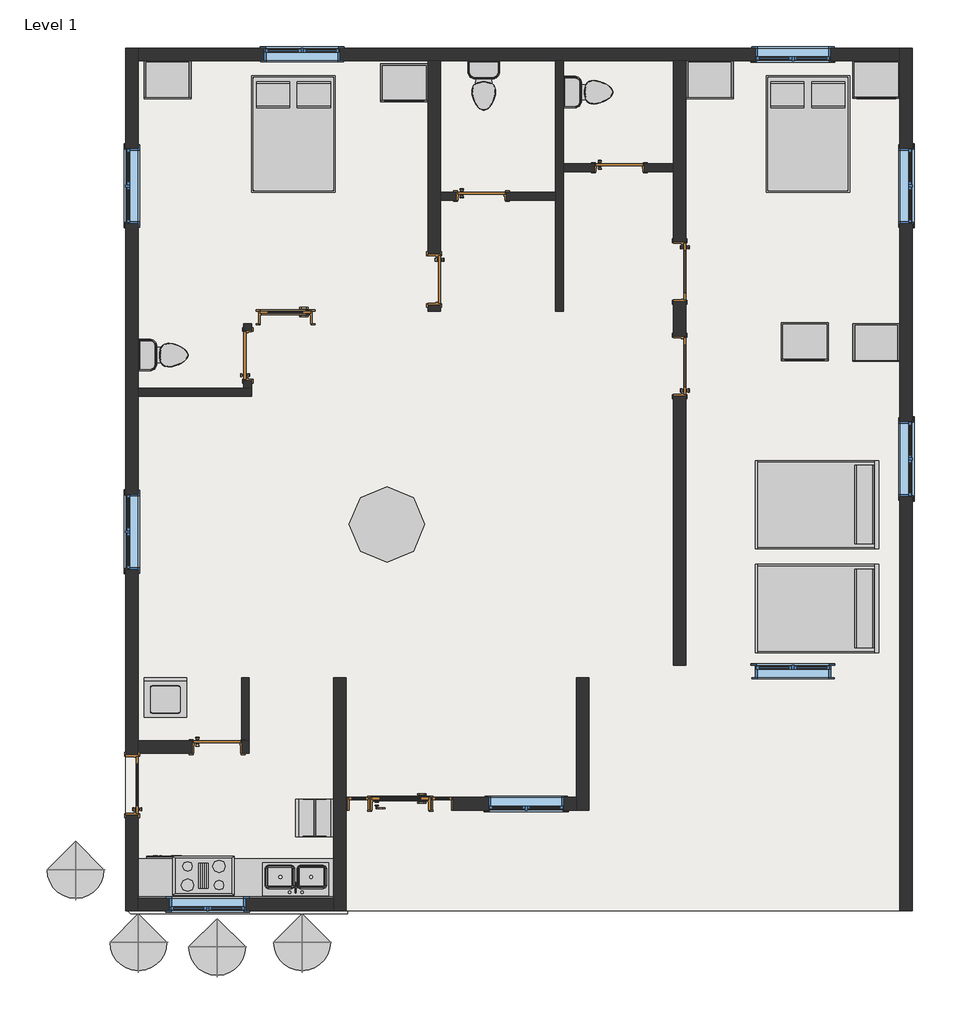
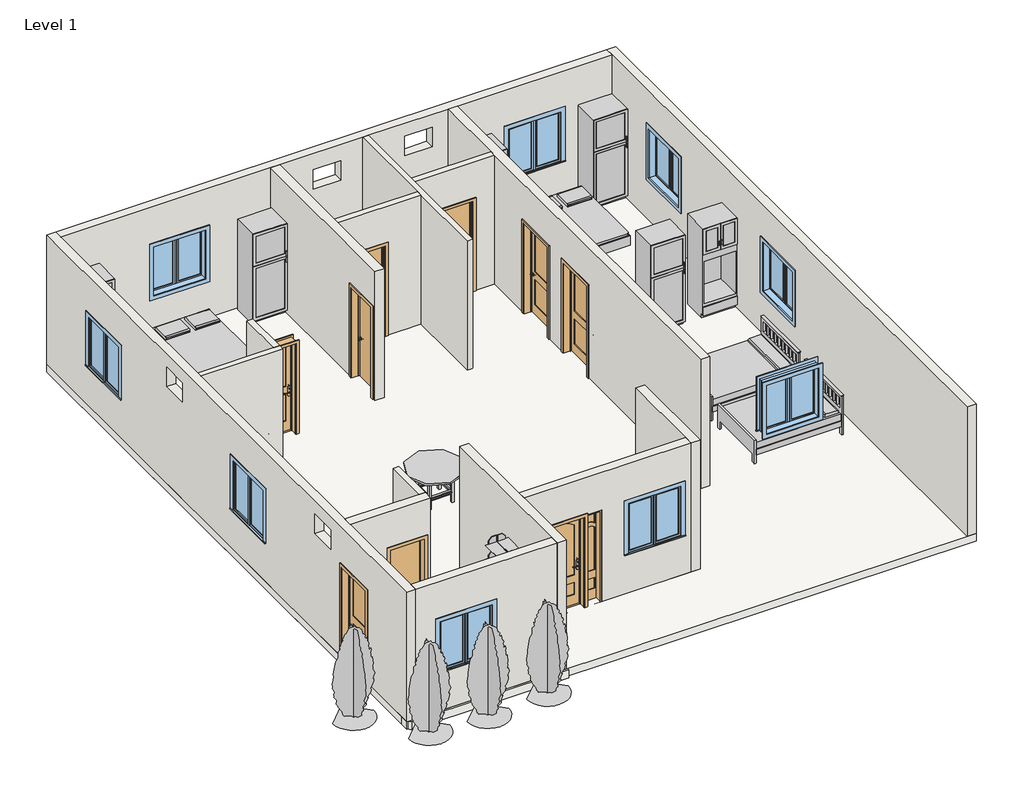
# One storey, incomplete: 16 walls, 13 doors, 12 furniture elements, 9 windows, 4 flow terminals, 4 geographic elements, 4 proxies, 3 slabs.
# Revit data of these elements (continued)
# Element 7 (IfcDoor, "32\" x 84\"") (continued)
#   Materials on its faces: "Cherry", "Aluminum", "Glass"
# Element 8 (IfcDoor, "36\" x 84\"")
#   Threshold Offset = 0' - 0 1/2"
#   Swing Angle = 90.00°
#   Door Offset = 0' - 0"
#   Threshold = yes
#   Exterior Trim = yes
#   Phase Created = New Construction
#   Materials on its faces: "Cherry", "Aluminum", "Glass"
# Elements 9, 10, 11 (IfcDoor, "Door-Interior-Single-2_Panel-Wood : 36\" x 84\"")
#   Swing Angle = 90.00°
#   Phase Created = New Construction
#   Materials on its faces: "Cherry", "Aluminum"
# Elements 12, 13, 14, 15 (IfcDoor, "Door-Interior-Single-Flush_Panel-Wood")
#   Swing Angle = 90.00°
#   Phase Created = New Construction
#   Materials on its faces: "Cherry", "Aluminum"
# Element 16 (IfcDoor, "Door-Interior-Single-Flush_Panel-Wood : 30\" x 84\"")
#   Swing Angle = 90.00°
#   Phase Created = New Construction
#   Materials on its faces: "Cherry", "Aluminum"
# Element 17 (IfcDoor, "Entry Door Handle : Standard")
#   Phase Created = New Construction
#   Materials on its faces: "Aluminum"
# Element 18 (IfcFlowTerminal, "Sink Kitchen-Double : 42\" x 21\"")
#   Mark = "1"
#   Phase Created = New Construction
#   Materials on its faces: "Steel, Polished"
# Element 19 (IfcFlowTerminal, "Toilet-Domestic-3D : Toilet-Domestic-3D")
#   Mark = "2"
#   Phase Created = New Construction
#   Materials on its faces: "Porcelain, Linen", "Laminate, Linen, Matte"
# Element 20 (IfcFlowTerminal, "Toilet-Domestic-3D : Toilet-Domestic-3D")
#   Mark = "3"
#   Phase Created = New Construction
#   Materials on its faces: "Porcelain, Linen", "Laminate, Linen, Matte"
# Element 21 (IfcFlowTerminal, "Toilet-Domestic-3D : Toilet-Domestic-3D")
#   Mark = "4"
#   Phase Created = New Construction
#   Materials on its faces: "Porcelain, Linen", "Laminate, Linen, Matte"
# Elements 22, 23 (IfcFurniture, "Bed-Box : Double 53\" x 74\"")
#   Phase Created = New Construction
#   Materials on its faces: "Birch", "Linen, White"
# Elements 24, 25 (IfcFurniture, "Bed-Shaker : Double 56\" x 78\"")
#   Phase Created = New Construction
#   Materials on its faces: "Birch", "Linen, White"
# Element 26 (IfcFurniture, "Counter Top w Sink : 24\" Depth")
#   Sink Opening Width = 3' - 3"
#   Sink Opening Depth = 1' - 3"
#   Sink Location To Wall = 0' - 6"
#   Sink Location = 2' - 0"
#   Length = 10' - 4"
#   Phase Created = New Construction
#   Materials on its faces: "Counter Top"
# Element 27 (IfcFurniture, "Table-Dining Round w Chairs : 36\" Diameter")
#   Phase Created = New Construction
#   Materials on its faces: "Pine", "Laminate, Linen, Matte"
# Elements 28, 29, 30 (IfcFurniture, "Tall Cabinet-2 Door-Built in : 30\"")
#   Phase Created = New Construction
#   Materials on its faces: "Cabinets", "Cabinets - Handles", "Glass"
# Elements 31, 32, 33 (IfcFurniture, "Tall Cabinet-Single Door(2) : 30\"")
#   Phase Created = New Construction
#   Materials on its faces: "Cabinets", "Cabinets - Handles"
# Elements 34, 35, 36, 37 (IfcGeographicElement, "RPC Tree - Conifer : Chinese Juniper - 7'")
#   Phase Created = New Construction
# Elements 38, 39, 40 (IfcSlab, "Generic - 12\"")
#   Height Offset From Level = 0' - 0"
#   Phase Created = New Construction
#   Materials on its faces: "Plywood, Sheathing"
# Elements 41, 42 (IfcWall)
#   Top Offset = 0' - 0"
#   Base Offset = 0' - 0"
#   Unconnected Height = 10' - 0"
#   wall height = 10' - 0"
#   Phase Created = New Construction
#   Base Constraint = Level 1
#   Materials on its faces: "Birch"
# Elements 43, 44, 45, 46 (IfcWall, "Generic - 5\"")
#   Top Offset = 0' - 0"
#   Base Offset = 0' - 0"
#   Unconnected Height = 10' - 0"
#   wall height = 10' - 0"
#   Phase Created = New Construction
#   Base Constraint = Level 1
#   Materials on its faces: "Default Wall"
# Elements 47, 48 (IfcWall, "Generic - 5\"")
#   Top Offset = 0' - 0"
#   Base Offset = 0' - 0"
#   wall height = 10' - 0"
#   Phase Created = New Construction
#   Base Constraint = Level 1
#   Top Constraint = Level 2
#   Materials on its faces: "Default Wall"
# Elements 49, 50, 52 (IfcWall, "Generic - 8\"")
#   Top Offset = 0' - 0"
#   Base Offset = 0' - 0"
#   Unconnected Height = 10' - 0"
#   wall height = 10' - 0"
#   Phase Created = New Construction
#   Base Constraint = Level 1
#   Materials on its faces: "Default Wall"
# Element 51 (IfcWall, "Generic - 8\"")
#   Top Offset = 0' - 0"
#   Base Offset = 0' - 0"
#   Unconnected Height = 10' - 0"
#   wall height = 10' - 0"
#   Phase Created = New Construction
#   Base Constraint = Level 1
#   Materials on its faces: "Default Wall", "Birch"
# Element 53 (IfcWall, "a")
#   Top Offset = 0' - 0"
#   Base Offset = 0' - 0"
#   Unconnected Height = 10' - 0"
#   wall height = 10' - 0"
#   Phase Created = New Construction
#   Base Constraint = Level 1
#   Materials on its faces: "Birch"
# Element 54 (IfcWall, "aw")
#   Top Offset = 0' - 0"
#   Base Offset = 0' - 0"
#   Unconnected Height = 10' - 0"
#   wall height = 10' - 0"
#   Phase Created = New Construction
#   Base Constraint = Level 1
#   Materials on its faces: "Birch"
# Elements 55, 56 (IfcWall, "dq")
#   Top Offset = 0' - 0"
#   Base Offset = 0' - 0"
#   Unconnected Height = 10' - 0"
#   wall height = 10' - 0"
#   Phase Created = New Construction
#   Base Constraint = Level 1
#   Materials on its faces: "Birch"
# Element 57 (IfcWindow, "Casement Dbl with Trim : 48\" x 48\"")
#   Mark = "3"
#   Phase Created = New Construction
#   Materials on its faces: "Sash", "Trim", "Glass"
# Element 58 (IfcWindow, "Casement Dbl with Trim : 48\" x 48\"")
#   Mark = "4"
#   Phase Created = New Construction
#   Materials on its faces: "Sash", "Trim", "Glass"
# Element 59 (IfcWindow, "Casement Dbl with Trim : 48\" x 48\"")
#   Mark = "2"
#   Phase Created = New Construction
#   Materials on its faces: "Sash", "Trim", "Glass"
# Element 60 (IfcWindow, "Casement Dbl with Trim : 48\" x 48\"")
#   Mark = "1"
#   Phase Created = New Construction
#   Materials on its faces: "Sash", "Trim", "Glass"
# Element 61 (IfcWindow, "Casement Dbl with Trim : 48\" x 48\"")
#   Mark = "7"
#   Phase Created = New Construction
#   Materials on its faces: "Sash", "Trim", "Glass"
# Element 62 (IfcWindow, "Casement Dbl with Trim : 48\" x 48\"")
#   Mark = "8"
#   Phase Created = New Construction
#   Materials on its faces: "Sash", "Trim", "Glass"
# Element 63 (IfcWindow, "Casement Dbl with Trim : 48\" x 48\"")
#   Mark = "6"
#   Phase Created = New Construction
#   Materials on its faces: "Sash", "Trim", "Glass"
# Element 64 (IfcWindow, "Casement Dbl with Trim : 48\" x 48\"")
#   Mark = "18"
#   Phase Created = New Construction
#   Materials on its faces: "Sash", "Trim", "Glass"
# Element 65 (IfcWindow, "Casement Dbl with Trim : 48\" x 48\"")
#   Mark = "5"
#   Phase Created = New Construction
#   Materials on its faces: "Sash", "Trim", "Glass"
# Materials
#   "Steel, Chrome Plated": class "Metal", colour RGB 17 17 17, transparency 0, Description = "Chromiuim plated steel", Cost = 0
#   "Steel, Polished": class "Metal", colour RGB 192 192 192, transparency 0, Description = "Polished steel", Cost = 0
#   "Steel, Paint Finish, Ivory, Glossy": class "Metal", colour RGB 247 247 239, transparency 0, Description = "Steel, paint finish, ivory, glossy", Cost = 0
#   "Plastic, Opaque Black": class "Plastic", colour RGB 0 0 0, transparency 0.7, Description = "Plastic, generic, opaque black", Cost = 0
#   "Steel, Paint Finish, Ivory, Matte": class "Metal", colour RGB 247 247 239, transparency 0, Description = "Steel, paint finish, ivory, matte", Cost = 0
#   "Cherry": class "Wood", colour RGB 226 177 128, transparency 0, Description = "Prunus Serotina", Cost = 0
#   "Glass": class "Glass", colour RGB 0 128 192, transparency 0.75, Description = "Soda Lime Glass", Cost = 0
#   "Aluminum": class "Metal", colour RGB 247 247 247, transparency 0, Description = "Aluminum 6061", Cost = 0
#   "Porcelain, Linen": class "Ceramic", colour RGB 249 239 230, transparency 0, Description = "Porcelain, linen", Cost = 0
#   "Laminate, Linen, Matte": class "Plastic", colour RGB 249 239 230, transparency 0, Description = "Plastic Laminate - Linen, Matte", Cost = 0
#   "Birch": class "Wood", colour RGB 224 178 126, transparency 0, Description = "Betula Alleghaniensis", Cost = 0
#   "Linen, White": class "Textile", colour RGB 247 247 239, transparency 0, Description = "Linen, white", Cost = 0
#   "Pine": class "Wood", colour RGB 223 192 134, transparency 0, Description = "Pinus Echinata", Cost = 0
#   "Cabinets - Handles": class "Metal", colour RGB 57 57 57, transparency 0
#   "Plywood, Sheathing": class "Wood", colour RGB 212 179 113, transparency 0, Description = "Plywood, sheathing grade", Cost = 0
#   "Sash": class "Wood", colour RGB 224 178 126, transparency 0
#   "Trim": class "Wood", colour RGB 224 178 126, transparency 0
#   "Counter Top": class "Wood", colour RGB 226 177 128, transparency 0
#   "Cabinets": colour RGB 249 249 249, transparency 0
#   "Default Wall": colour RGB 128 128 128, transparency 0
